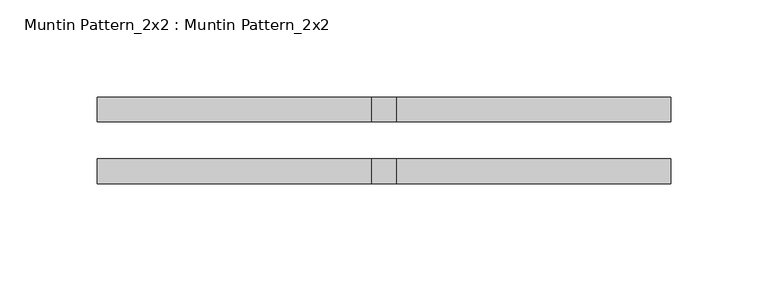
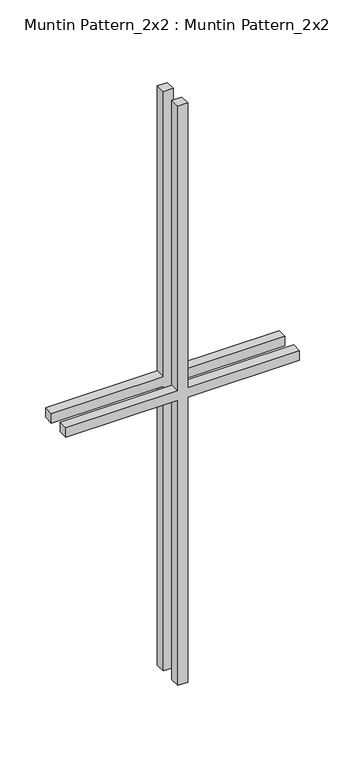
"""IFC4 building model written with IfcOpenShell, lengths in millimetres: proxy geometry, Muntin Pattern_2x2 : Muntin Pattern_2x2."""

from ifc_helpers import new_model, si_unit, frame, origin, place, context, project, spatial, polyline, outline, extrude, source, transform, mapped, element, save


def muntin_pattern_2x2_muntin_pattern_2x2_3e0ecaf2(model_context):
    return source(origin(), model_context, "Body", "SweptSolid", [
        extrude(outline(polyline([(393.7, -6.35), (393.7, -147.6375), (381.0, -147.6375), (381.0, -6.35), (0.0, -6.35), (0.0, 6.35), (381.0, 6.35), (381.0, 147.6375), (393.7, 147.6375), (393.7, 6.35), (774.7, 6.35), (774.7, -6.35), (393.7, -6.35)])), frame((0.0, -22.225, 0.0), z_axis=(0.0, 1.0, 0.0), x_axis=(0.0, 0.0, 1.0)), (0.0, 0.0, 1.0), 12.7),
        extrude(outline(polyline([(393.7, -6.35), (393.7, -147.6375), (381.0, -147.6375), (381.0, -6.35), (0.0, -6.35), (0.0, 6.35), (381.0, 6.35), (381.0, 147.6375), (393.7, 147.6375), (393.7, 6.35), (774.7, 6.35), (774.7, -6.35), (393.7, -6.35)])), frame((0.0, 9.525, 0.0), z_axis=(0.0, 1.0, 0.0), x_axis=(0.0, 0.0, 1.0)), (0.0, 0.0, 1.0), 12.7),
    ])


if __name__ == "__main__":
    model = new_model("IFC4")
    model_context = context("Model", 3, world=origin())
    ifc_project = project(units=[si_unit("LENGTHUNIT", "METRE", prefix="MILLI")], contexts=[model_context])
    site = spatial("IfcSite", under=ifc_project)
    building = spatial("IfcBuilding", under=site)
    placement = place(None, origin())
    muntin_pattern_2x2_muntin_pattern_2x2_shape = muntin_pattern_2x2_muntin_pattern_2x2_3e0ecaf2(model_context)
    element("IfcBuildingElementProxy", 1, Name="Muntin Pattern_2x2 : Muntin Pattern_2x2", ObjectType="Muntin Pattern_2x2 : Muntin Pattern_2x2", at=placement, inside=building, context=model_context, shape_type="MappedRepresentation", body=[
        mapped(muntin_pattern_2x2_muntin_pattern_2x2_shape, transform((0.0, 0.0, 0.0), x_axis=(1.0, 0.0, 0.0), y_axis=(0.0, 1.0, 0.0), z_axis=(0.0, 0.0, 1.0))),
    ])
    save(model, "model.ifc")

# Revit data of these elements
# Type "Muntin Pattern_2x2 : Muntin Pattern_2x2"
#   Width [instance default] = 4 ft
#   Thickness = 0.041667 ft
#   Height [instance default] = 4 ft
#   Distance = 0.0625 ft
#   Interior Material [instance default] = none
#   Exterior Material [instance default] = none
#   Default Elevation = 0
# Element 1 (IfcBuildingElementProxy, "Muntin Pattern_2x2 : Muntin Pattern_2x2")
#   Width = 0.96875 ft
#   Height = 2.541667 ft
#   Interior Material = Wood - Stained
#   Exterior Material = Clad - White
#   Materials on its faces: "Clad - White", "Wood - Stained"
# Materials
#   "Clad - White": class "Wood", colour RGB 242 242 238, transparency 0, Cost = 0
#   "Wood - Stained": class "Wood", colour RGB 224 178 126, transparency 0, Cost = 0
